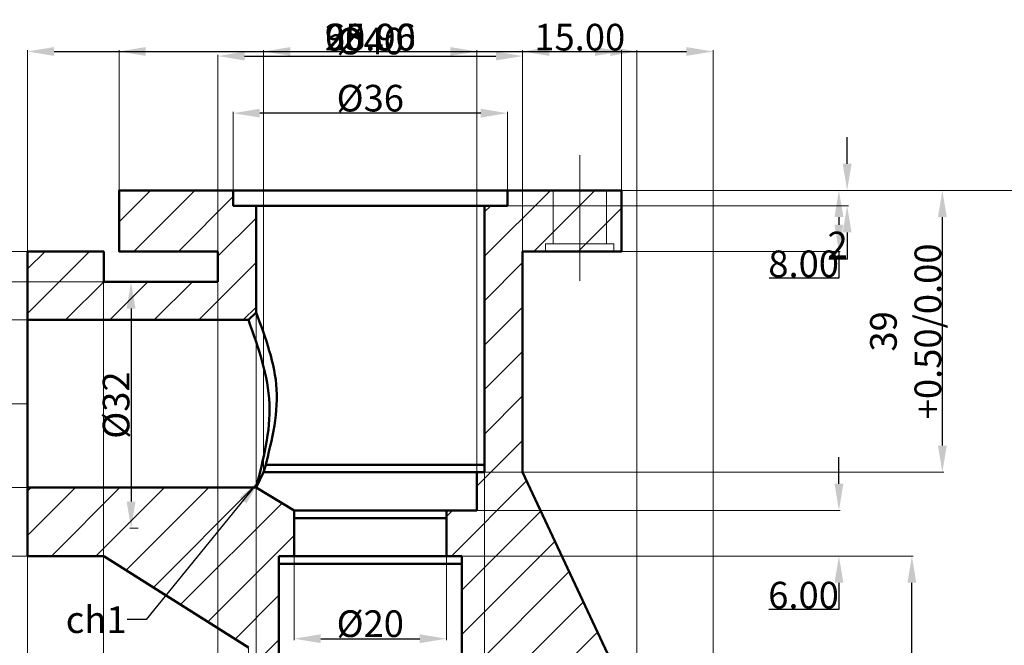
# Model space of a CAD drawing. Units: millimetres. Extents: x 75 to 489, y 21 to 350.
# Tile 4 of 5: x 142 to 271, y 268 to 350. Entities that reach past the tile are written whole.
import ezdxf

# ---------------------------------------------------------------- set-up
doc = ezdxf.new("R2010")
doc.units = ezdxf.units.MM
doc.header["$MEASUREMENT"] = 0
doc.linetypes.add('CENTER', pattern=[50.8, 31.75, -6.35, 6.35, -6.35])
for name, color, linetype, lineweight in [('M-CNTR', 1, 'CENTER', 18), ('M-DIMS', 2, 'Continuous', 25), ('M-HATC', 8, 'Continuous', 18), ('M-OUTL', 7, 'Continuous', 50), ('M-TEXT', 7, 'Continuous', 25), ('M-THRD', 3, 'Continuous', 18)]:
    doc.layers.add(name, color=color, linetype=linetype, lineweight=lineweight)
doc.styles.get("Standard").update_dxf_attribs({"font": 'arial.ttf'})
doc.dimstyles.get("Standard").update_dxf_attribs({"dimtxt": 3.5, "dimasz": 3.5, "dimexe": 0.18, "dimexo": 0.0625, "dimgap": 0.09, "dimtad": 1, "dimtoh": 1, "dimdec": 0, "dimzin": 0, "dimdsep": 46, "dimtxsty": 'Standard', "dimcen": 0.09, "dimclrd": 2, "dimclre": 251, "dimadec": 0, "dimazin": 0, "dimtfac": 1, "dimtdec": 0, "dimtofl": 0, "dimtmove": 0, "dimatfit": 3, "dimfxl": 1, "dimtolj": 1, "dimtzin": 0, "dimlwe": 5, "dimarcsym": 0})

# ---------------------------------------------------------------- blocks, each defined once
blk = doc.blocks.new('*D21')
at = {"layer": 'Defpoints', "color": 0, "transparency": 16777216}
for p in [(169.9, 337.5), (169.9, 327.35), (205.9, 327.35)]:
    blk.add_point(p, dxfattribs=at)
at = {"layer": 'M-DIMS', "color": 0, "lineweight": 5, "transparency": 16777216}
for p, q in [((169.9, 327.41), (169.9, 337.68)), ((205.9, 327.41), (205.9, 337.68))]:
    blk.add_line(p, q, dxfattribs=at)
at = {"layer": 'M-DIMS', "color": 0, "lineweight": -2, "transparency": 16777216}
blk.add_line((202.4, 337.5), (173.4, 337.5), dxfattribs=at)
at = {"layer": 'M-DIMS', "color": 0, "transparency": 16777216}
for points in [[(173.4, 338.08), (173.4, 336.92), (169.9, 337.5)], [(202.4, 338.08), (202.4, 336.92), (205.9, 337.5)]]:
    blk.add_solid(points, dxfattribs=at)
at = {"layer": 'M-DIMS', "color": 0, "transparency": 16777216, "insert": (187.9, 339.47), "char_height": 3.5, "attachment_point": 5}
blk.add_mtext('\\A1;%%C36', dxfattribs=at)
blk = doc.blocks.new('*D22')
at = {"layer": 'Defpoints', "color": 0, "transparency": 16777216}
for p in [(207.9, 345), (167.9, 319.35), (207.9, 319.35)]:
    blk.add_point(p, dxfattribs=at)
at = {"layer": 'M-DIMS', "color": 0, "lineweight": 5, "transparency": 16777216}
for p, q in [((167.9, 319.41), (167.9, 345.18)), ((207.9, 319.41), (207.9, 345.18))]:
    blk.add_line(p, q, dxfattribs=at)
at = {"layer": 'M-DIMS', "color": 0, "lineweight": -2, "transparency": 16777216}
blk.add_line((171.4, 345), (204.4, 345), dxfattribs=at)
at = {"layer": 'M-DIMS', "color": 0, "transparency": 16777216}
for points in [[(171.4, 345.58), (171.4, 344.42), (167.9, 345)], [(204.4, 345.58), (204.4, 344.42), (207.9, 345)]]:
    blk.add_solid(points, dxfattribs=at)
at = {"layer": 'M-DIMS', "color": 0, "transparency": 16777216, "insert": (187.9, 346.97), "char_height": 3.5, "attachment_point": 5}
blk.add_mtext('\\A1;%%C40', dxfattribs=at)
blk = doc.blocks.new('*D23')
at = {"layer": 'Defpoints', "color": 0, "transparency": 16777216}
for p in [(157.5, 315.35), (156.5, 283), (157.5, 283)]:
    blk.add_point(p, dxfattribs=at)
at = {"layer": 'M-DIMS', "color": 0, "lineweight": 5, "transparency": 16777216}
for p, q in [((157.44, 315.35), (156.32, 315.35)), ((157.44, 283), (156.32, 283))]:
    blk.add_line(p, q, dxfattribs=at)
at = {"layer": 'M-DIMS', "color": 0, "lineweight": -2, "transparency": 16777216}
blk.add_line((156.5, 311.85), (156.5, 286.5), dxfattribs=at)
at = {"layer": 'M-DIMS', "color": 0, "transparency": 16777216}
for points in [[(155.92, 311.85), (157.08, 311.85), (156.5, 315.35)], [(155.92, 286.5), (157.08, 286.5), (156.5, 283)]]:
    blk.add_solid(points, dxfattribs=at)
at = {"layer": 'M-DIMS', "color": 0, "transparency": 16777216, "insert": (154.53, 299.17), "char_height": 3.5, "attachment_point": 5, "rotation": 90}
blk.add_mtext('\\A1;%%C32', dxfattribs=at)
blk = doc.blocks.new('*D24')
at = {"layer": 'Defpoints', "color": 0, "transparency": 16777216}
for p in [(133, 310.35), (142.9, 310.35), (142.9, 288.35)]:
    blk.add_point(p, dxfattribs=at)
at = {"layer": 'M-DIMS', "color": 0, "lineweight": 5, "transparency": 16777216}
for p, q in [((142.84, 310.35), (132.82, 310.35)), ((142.84, 288.35), (132.82, 288.35))]:
    blk.add_line(p, q, dxfattribs=at)
at = {"layer": 'M-DIMS', "color": 0, "lineweight": -2, "transparency": 16777216}
blk.add_line((133, 291.85), (133, 306.85), dxfattribs=at)
at = {"layer": 'M-DIMS', "color": 0, "transparency": 16777216}
for points in [[(132.42, 306.85), (133.58, 306.85), (133, 310.35)], [(132.42, 291.85), (133.58, 291.85), (133, 288.35)]]:
    blk.add_solid(points, dxfattribs=at)
at = {"layer": 'M-DIMS', "color": 0, "transparency": 16777216, "insert": (131.03, 299.35), "char_height": 3.5, "attachment_point": 5, "rotation": 90}
blk.add_mtext('\\A1;%%C22', dxfattribs=at)
blk = doc.blocks.new('*D25')
at = {"layer": 'Defpoints', "color": 0, "transparency": 16777216}
for p in [(142.9, 299.35), (125.5, 241.35), (232.9, 241.35)]:
    blk.add_point(p, dxfattribs=at)
at = {"layer": 'M-DIMS', "color": 0, "lineweight": 5, "transparency": 16777216}
for p, q in [((142.84, 299.35), (125.32, 299.35)), ((232.84, 241.35), (125.32, 241.35))]:
    blk.add_line(p, q, dxfattribs=at)
at = {"layer": 'M-DIMS', "color": 0, "lineweight": -2, "transparency": 16777216}
blk.add_line((125.5, 295.85), (125.5, 244.85), dxfattribs=at)
at = {"layer": 'M-DIMS', "color": 0, "transparency": 16777216}
for points in [[(124.92, 295.85), (126.08, 295.85), (125.5, 299.35)], [(124.92, 244.85), (126.08, 244.85), (125.5, 241.35)]]:
    blk.add_solid(points, dxfattribs=at)
at = {"layer": 'M-DIMS', "color": 0, "transparency": 16777216, "insert": (123.62, 270.35), "char_height": 3.5, "attachment_point": 5, "rotation": 90}
blk.add_mtext('\\A1;58', dxfattribs=at)
blk = doc.blocks.new('*D26')
at = {"layer": 'Defpoints', "color": 0, "transparency": 16777216}
for p in [(117, 299.35), (142.9, 299.35), (155.4, 209.35)]:
    blk.add_point(p, dxfattribs=at)
at = {"layer": 'M-DIMS', "color": 0, "lineweight": 5, "transparency": 16777216}
for p, q in [((142.84, 299.35), (116.82, 299.35)), ((155.34, 209.35), (116.82, 209.35))]:
    blk.add_line(p, q, dxfattribs=at)
at = {"layer": 'M-DIMS', "color": 0, "lineweight": -2, "transparency": 16777216}
blk.add_line((117, 212.85), (117, 295.85), dxfattribs=at)
at = {"layer": 'M-DIMS', "color": 0, "transparency": 16777216}
for points in [[(116.42, 295.85), (117.58, 295.85), (117, 299.35)], [(116.42, 212.85), (117.58, 212.85), (117, 209.35)]]:
    blk.add_solid(points, dxfattribs=at)
at = {"layer": 'M-DIMS', "color": 0, "transparency": 16777216, "insert": (115.12, 254.35), "char_height": 3.5, "attachment_point": 5, "rotation": 90}
blk.add_mtext('\\A1;90', dxfattribs=at)
blk = doc.blocks.new('*D31')
at = {"layer": 'Defpoints', "color": 0, "transparency": 16777216}
for p in [(199.9, 279.35), (259, 279.35), (220.4, 209.35)]:
    blk.add_point(p, dxfattribs=at)
at = {"layer": 'M-DIMS', "color": 0, "lineweight": 5, "transparency": 16777216}
for p, q in [((199.97, 279.35), (259.18, 279.35)), ((220.47, 209.35), (259.18, 209.35))]:
    blk.add_line(p, q, dxfattribs=at)
at = {"layer": 'M-DIMS', "color": 0, "lineweight": -2, "transparency": 16777216}
blk.add_line((259, 212.85), (259, 275.85), dxfattribs=at)
at = {"layer": 'M-DIMS', "color": 0, "transparency": 16777216}
for points in [[(258.42, 275.85), (259.58, 275.85), (259, 279.35)], [(258.42, 212.85), (259.58, 212.85), (259, 209.35)]]:
    blk.add_solid(points, dxfattribs=at)
at = {"layer": 'M-DIMS', "color": 0, "transparency": 16777216, "insert": (257.12, 244.35), "char_height": 3.5, "attachment_point": 5, "rotation": 90}
blk.add_mtext('\\A1;70', dxfattribs=at)
blk = doc.blocks.new('*D32')
at = {"layer": 'Defpoints', "color": 0, "transparency": 16777216}
for p in [(177.9, 279.35), (197.9, 279.35), (197.9, 268.5)]:
    blk.add_point(p, dxfattribs=at)
at = {"layer": 'M-DIMS', "color": 0, "lineweight": 5, "transparency": 16777216}
for p, q in [((177.9, 279.28), (177.9, 268.32)), ((197.9, 279.28), (197.9, 268.32))]:
    blk.add_line(p, q, dxfattribs=at)
at = {"layer": 'M-DIMS', "color": 0, "lineweight": -2, "transparency": 16777216}
blk.add_line((181.4, 268.5), (194.4, 268.5), dxfattribs=at)
at = {"layer": 'M-DIMS', "color": 0, "transparency": 16777216}
for points in [[(181.4, 269.08), (181.4, 267.92), (177.9, 268.5)], [(194.4, 269.08), (194.4, 267.92), (197.9, 268.5)]]:
    blk.add_solid(points, dxfattribs=at)
at = {"layer": 'M-DIMS', "color": 0, "transparency": 16777216, "insert": (187.9, 270.47), "char_height": 3.5, "attachment_point": 5}
blk.add_mtext('\\A1;%%C20', dxfattribs=at)
blk = doc.blocks.new('*D33')
at = {"layer": 'Defpoints', "color": 0, "transparency": 16777216}
for p in [(205.9, 327.35), (205.9, 325.35), (250.5, 325.35)]:
    blk.add_point(p, dxfattribs=at)
at = {"layer": 'M-DIMS', "color": 0, "lineweight": -2, "transparency": 16777216}
for p, q in [((250.5, 330.85), (250.5, 334.35)), ((250.5, 321.85), (250.5, 318.35)), ((250.5, 318.35), (248.09, 318.35))]:
    blk.add_line(p, q, dxfattribs=at)
at = {"layer": 'M-DIMS', "color": 0, "lineweight": 5, "transparency": 16777216}
for p, q in [((205.97, 327.35), (250.68, 327.35)), ((205.97, 325.35), (250.68, 325.35))]:
    blk.add_line(p, q, dxfattribs=at)
at = {"layer": 'M-DIMS', "color": 0, "transparency": 16777216}
for points in [[(249.92, 330.85), (251.08, 330.85), (250.5, 327.35)], [(249.92, 321.85), (251.08, 321.85), (250.5, 325.35)]]:
    blk.add_solid(points, dxfattribs=at)
at = {"layer": 'M-DIMS', "color": 0, "transparency": 16777216, "insert": (249.25, 320.19), "char_height": 3.5, "attachment_point": 5}
blk.add_mtext('\\A1;2', dxfattribs=at)
blk = doc.blocks.new('*D34')
at = {"layer": 'Defpoints', "color": 0, "transparency": 16777216}
for p in [(205.9, 327.35), (263, 327.35), (202.9, 290.35)]:
    blk.add_point(p, dxfattribs=at)
at = {"layer": 'M-DIMS', "color": 0, "lineweight": 5, "transparency": 16777216}
for p, q in [((205.97, 327.35), (263.18, 327.35)), ((202.97, 290.35), (263.18, 290.35))]:
    blk.add_line(p, q, dxfattribs=at)
at = {"layer": 'M-DIMS', "color": 0, "lineweight": -2, "transparency": 16777216}
blk.add_line((263, 293.85), (263, 323.85), dxfattribs=at)
at = {"layer": 'M-DIMS', "color": 0, "transparency": 16777216}
for points in [[(262.42, 323.85), (263.58, 323.85), (263, 327.35)], [(262.42, 293.85), (263.58, 293.85), (263, 290.35)]]:
    blk.add_solid(points, dxfattribs=at)
at = {"layer": 'M-DIMS', "color": 0, "transparency": 16777216, "insert": (258.18, 308.85), "char_height": 3.5, "attachment_point": 5, "rotation": 90}
blk.add_mtext('\\A1;39\\P+0.50/0.00', dxfattribs=at)
blk = doc.blocks.new('*D35')
at = {"layer": 'Defpoints', "color": 0, "transparency": 16777216}
for p in [(220.88, 327.35), (259, 209.35), (279.5, 209.35)]:
    blk.add_point(p, dxfattribs=at)
at = {"layer": 'M-DIMS', "color": 0, "lineweight": 5, "transparency": 16777216}
for p, q in [((220.95, 327.35), (279.68, 327.35)), ((259.06, 209.35), (279.68, 209.35))]:
    blk.add_line(p, q, dxfattribs=at)
at = {"layer": 'M-DIMS', "color": 0, "lineweight": -2, "transparency": 16777216}
blk.add_line((279.5, 323.85), (279.5, 212.85), dxfattribs=at)
at = {"layer": 'M-DIMS', "color": 0, "transparency": 16777216}
for points in [[(278.92, 323.85), (280.08, 323.85), (279.5, 327.35)], [(278.92, 212.85), (280.08, 212.85), (279.5, 209.35)]]:
    blk.add_solid(points, dxfattribs=at)
at = {"layer": 'M-DIMS', "color": 0, "transparency": 16777216, "insert": (277.62, 268.35), "char_height": 3.5, "attachment_point": 5, "rotation": 90}
blk.add_mtext('\\A1;118', dxfattribs=at)
blk = doc.blocks.new('*D44')
at = {"layer": 'Defpoints', "color": 0, "transparency": 16777216}
for p in [(232.9, 345.6), (142.9, 319.35), (232.9, 258.35)]:
    blk.add_point(p, dxfattribs=at)
at = {"layer": 'M-DIMS', "color": 251, "lineweight": 5, "transparency": 16777216}
for p, q in [((142.9, 319.41), (142.9, 345.78)), ((232.9, 258.41), (232.9, 345.78))]:
    blk.add_line(p, q, dxfattribs=at)
at = {"layer": 'M-DIMS', "color": 2, "lineweight": -2, "transparency": 16777216}
blk.add_line((146.4, 345.6), (229.4, 345.6), dxfattribs=at)
at = {"layer": 'M-DIMS', "color": 2, "transparency": 16777216}
for points in [[(146.4, 346.18), (146.4, 345.02), (142.9, 345.6)], [(229.4, 346.18), (229.4, 345.02), (232.9, 345.6)]]:
    blk.add_solid(points, dxfattribs=at)
at = {"layer": 'M-DIMS', "color": 0, "transparency": 16777216, "insert": (187.9, 347.48), "char_height": 3.5, "attachment_point": 5}
blk.add_mtext('\\A1;90.00', dxfattribs=at)
blk = doc.blocks.new('*D45')
at = {"layer": 'Defpoints', "color": 0, "transparency": 16777216}
for p in [(220.88, 345.6), (154.92, 327.35), (220.88, 327.35)]:
    blk.add_point(p, dxfattribs=at)
at = {"layer": 'M-DIMS', "color": 251, "lineweight": 5, "transparency": 16777216}
for p, q in [((154.92, 327.41), (154.92, 345.78)), ((220.88, 327.41), (220.88, 345.78))]:
    blk.add_line(p, q, dxfattribs=at)
at = {"layer": 'M-DIMS', "color": 2, "lineweight": -2, "transparency": 16777216}
blk.add_line((158.42, 345.6), (217.38, 345.6), dxfattribs=at)
at = {"layer": 'M-DIMS', "color": 2, "transparency": 16777216}
for points in [[(158.42, 346.18), (158.42, 345.02), (154.92, 345.6)], [(217.38, 346.18), (217.38, 345.02), (220.88, 345.6)]]:
    blk.add_solid(points, dxfattribs=at)
at = {"layer": 'M-DIMS', "color": 0, "transparency": 16777216, "insert": (187.9, 347.48), "char_height": 3.5, "attachment_point": 5}
blk.add_mtext('\\A1;65.96', dxfattribs=at)
blk = doc.blocks.new('*D46')
at = {"layer": 'Defpoints', "color": 0, "transparency": 16777216}
for p in [(220.88, 327.35), (220.88, 319.35), (249.42, 319.35)]:
    blk.add_point(p, dxfattribs=at)
at = {"layer": 'M-DIMS', "color": 251, "lineweight": 5, "transparency": 16777216}
for p, q in [((220.95, 327.35), (249.6, 327.35)), ((220.95, 319.35), (249.6, 319.35))]:
    blk.add_line(p, q, dxfattribs=at)
at = {"layer": 'M-DIMS', "color": 2, "lineweight": -2, "transparency": 16777216}
for p, q in [((249.42, 323.85), (249.42, 322.85)), ((249.42, 319.35), (249.42, 315.85)), ((249.42, 315.85), (240.25, 315.85))]:
    blk.add_line(p, q, dxfattribs=at)
at = {"layer": 'M-DIMS', "color": 2, "transparency": 16777216}
for points in [[(248.84, 323.85), (250.01, 323.85), (249.42, 327.35)], [(248.84, 322.85), (250.01, 322.85), (249.42, 319.35)]]:
    blk.add_solid(points, dxfattribs=at)
at = {"layer": 'M-DIMS', "color": 0, "transparency": 16777216, "insert": (244.79, 317.72), "char_height": 3.5, "attachment_point": 5}
blk.add_mtext('\\A1;8.00', dxfattribs=at)
blk = doc.blocks.new('*D49')
at = {"layer": 'Defpoints', "color": 0, "transparency": 16777216}
for p in [(142.9, 319.35), (84.4, 279.35), (142.9, 279.35)]:
    blk.add_point(p, dxfattribs=at)
at = {"layer": 'M-DIMS', "color": 251, "lineweight": 5, "transparency": 16777216}
for p, q in [((142.84, 319.35), (84.22, 319.35)), ((142.84, 279.35), (84.22, 279.35))]:
    blk.add_line(p, q, dxfattribs=at)
at = {"layer": 'M-DIMS', "color": 2, "lineweight": -2, "transparency": 16777216}
blk.add_line((84.4, 315.85), (84.4, 282.85), dxfattribs=at)
at = {"layer": 'M-DIMS', "color": 2, "transparency": 16777216}
for points in [[(83.82, 315.85), (84.98, 315.85), (84.4, 319.35)], [(83.82, 282.85), (84.98, 282.85), (84.4, 279.35)]]:
    blk.add_solid(points, dxfattribs=at)
at = {"layer": 'M-DIMS', "color": 0, "transparency": 16777216, "insert": (82.52, 299.35), "char_height": 3.5, "attachment_point": 5, "rotation": 90}
blk.add_mtext('\\A1;40.00', dxfattribs=at)
blk = doc.blocks.new('*D50')
at = {"layer": 'Defpoints', "color": 0, "transparency": 16777216}
for p in [(142.9, 279.35), (152.9, 279.35), (152.9, 189.4)]:
    blk.add_point(p, dxfattribs=at)
at = {"layer": 'M-DIMS', "color": 251, "lineweight": 5, "transparency": 16777216}
for p, q in [((142.9, 279.28), (142.9, 189.22)), ((152.9, 279.28), (152.9, 189.22))]:
    blk.add_line(p, q, dxfattribs=at)
at = {"layer": 'M-DIMS', "color": 2, "lineweight": -2, "transparency": 16777216}
for p, q in [((146.4, 189.4), (149.4, 189.4)), ((152.9, 189.4), (168.05, 189.4))]:
    blk.add_line(p, q, dxfattribs=at)
at = {"layer": 'M-DIMS', "color": 2, "transparency": 16777216}
for points in [[(146.4, 189.98), (146.4, 188.82), (142.9, 189.4)], [(149.4, 189.98), (149.4, 188.82), (152.9, 189.4)]]:
    blk.add_solid(points, dxfattribs=at)
at = {"layer": 'M-DIMS', "color": 0, "transparency": 16777216, "insert": (162.23, 191.28), "char_height": 3.5, "attachment_point": 5}
blk.add_mtext('\\A1;10.00', dxfattribs=at)
blk = doc.blocks.new('*D51')
at = {"layer": 'Defpoints', "color": 0, "transparency": 16777216}
for p in [(142.9, 279.35), (171.9, 267.35), (171.9, 189.4)]:
    blk.add_point(p, dxfattribs=at)
at = {"layer": 'M-DIMS', "color": 251, "lineweight": 5, "transparency": 16777216}
for p, q in [((142.9, 279.28), (142.9, 189.22)), ((171.9, 267.28), (171.9, 189.22))]:
    blk.add_line(p, q, dxfattribs=at)
at = {"layer": 'M-DIMS', "color": 2, "lineweight": -2, "transparency": 16777216}
blk.add_line((146.4, 189.4), (168.4, 189.4), dxfattribs=at)
at = {"layer": 'M-DIMS', "color": 2, "transparency": 16777216}
for points in [[(146.4, 189.98), (146.4, 188.82), (142.9, 189.4)], [(168.4, 189.98), (168.4, 188.82), (171.9, 189.4)]]:
    blk.add_solid(points, dxfattribs=at)
at = {"layer": 'M-DIMS', "color": 0, "transparency": 16777216, "insert": (157.4, 191.28), "char_height": 3.5, "attachment_point": 5}
blk.add_mtext('\\A1;29.00', dxfattribs=at)
blk = doc.blocks.new('*D52')
at = {"layer": 'Defpoints', "color": 0, "transparency": 16777216}
for p in [(222.9, 345.6), (207.9, 290.35), (222.9, 258.35)]:
    blk.add_point(p, dxfattribs=at)
at = {"layer": 'M-DIMS', "color": 251, "lineweight": 5, "transparency": 16777216}
for p, q in [((207.9, 290.41), (207.9, 345.78)), ((222.9, 258.41), (222.9, 345.78))]:
    blk.add_line(p, q, dxfattribs=at)
at = {"layer": 'M-DIMS', "color": 2, "lineweight": -2, "transparency": 16777216}
blk.add_line((211.4, 345.6), (219.4, 345.6), dxfattribs=at)
at = {"layer": 'M-DIMS', "color": 2, "transparency": 16777216}
for points in [[(211.4, 346.18), (211.4, 345.02), (207.9, 345.6)], [(219.4, 346.18), (219.4, 345.02), (222.9, 345.6)]]:
    blk.add_solid(points, dxfattribs=at)
at = {"layer": 'M-DIMS', "color": 0, "transparency": 16777216, "insert": (215.4, 347.48), "char_height": 3.5, "attachment_point": 5}
blk.add_mtext('\\A1;15.00', dxfattribs=at)
blk = doc.blocks.new('*D53')
at = {"layer": 'Defpoints', "color": 0, "transparency": 16777216}
for p in [(152.9, 315.35), (167.9, 315.35), (167.9, 189.4)]:
    blk.add_point(p, dxfattribs=at)
at = {"layer": 'M-DIMS', "color": 251, "lineweight": 5, "transparency": 16777216}
for p, q in [((152.9, 315.28), (152.9, 189.22)), ((167.9, 315.28), (167.9, 189.22))]:
    blk.add_line(p, q, dxfattribs=at)
at = {"layer": 'M-DIMS', "color": 2, "lineweight": -2, "transparency": 16777216}
blk.add_line((156.4, 189.4), (164.4, 189.4), dxfattribs=at)
at = {"layer": 'M-DIMS', "color": 2, "transparency": 16777216}
for points in [[(156.4, 189.98), (156.4, 188.82), (152.9, 189.4)], [(164.4, 189.98), (164.4, 188.82), (167.9, 189.4)]]:
    blk.add_solid(points, dxfattribs=at)
at = {"layer": 'M-DIMS', "color": 0, "transparency": 16777216, "insert": (160.4, 191.28), "char_height": 3.5, "attachment_point": 5}
blk.add_mtext('\\A1;15.00', dxfattribs=at)
blk = doc.blocks.new('*D57')
at = {"layer": 'Defpoints', "color": 0, "transparency": 16777216}
for p in [(172.9, 325.35), (202.9, 325.35), (202.9, 189.4)]:
    blk.add_point(p, dxfattribs=at)
at = {"layer": 'M-DIMS', "color": 251, "lineweight": 5, "transparency": 16777216}
for p, q in [((172.9, 325.28), (172.9, 189.22)), ((202.9, 325.28), (202.9, 189.22))]:
    blk.add_line(p, q, dxfattribs=at)
at = {"layer": 'M-DIMS', "color": 2, "lineweight": -2, "transparency": 16777216}
blk.add_line((176.4, 189.4), (199.4, 189.4), dxfattribs=at)
at = {"layer": 'M-DIMS', "color": 2, "transparency": 16777216}
for points in [[(176.4, 189.98), (176.4, 188.82), (172.9, 189.4)], [(199.4, 189.98), (199.4, 188.82), (202.9, 189.4)]]:
    blk.add_solid(points, dxfattribs=at)
at = {"layer": 'M-DIMS', "color": 0, "transparency": 16777216, "insert": (187.9, 191.28), "char_height": 3.5, "attachment_point": 5}
blk.add_mtext('\\A1;30.00', dxfattribs=at)
blk = doc.blocks.new('*D58')
at = {"layer": 'Defpoints', "color": 0, "transparency": 16777216}
for p in [(201.9, 345.6), (173.9, 290.35), (201.9, 290.35)]:
    blk.add_point(p, dxfattribs=at)
at = {"layer": 'M-DIMS', "color": 251, "lineweight": 5, "transparency": 16777216}
for p, q in [((173.9, 290.41), (173.9, 345.78)), ((201.9, 290.41), (201.9, 345.78))]:
    blk.add_line(p, q, dxfattribs=at)
at = {"layer": 'M-DIMS', "color": 2, "lineweight": -2, "transparency": 16777216}
blk.add_line((177.4, 345.6), (198.4, 345.6), dxfattribs=at)
at = {"layer": 'M-DIMS', "color": 2, "transparency": 16777216}
for points in [[(177.4, 346.18), (177.4, 345.02), (173.9, 345.6)], [(198.4, 346.18), (198.4, 345.02), (201.9, 345.6)]]:
    blk.add_solid(points, dxfattribs=at)
at = {"layer": 'M-DIMS', "color": 0, "transparency": 16777216, "insert": (187.9, 347.48), "char_height": 3.5, "attachment_point": 5}
blk.add_mtext('\\A1;28.00', dxfattribs=at)
blk = doc.blocks.new('*D59')
at = {"layer": 'Defpoints', "color": 0, "transparency": 16777216}
for p in [(197.9, 285.35), (197.9, 279.35), (249.42, 279.35)]:
    blk.add_point(p, dxfattribs=at)
at = {"layer": 'M-DIMS', "color": 2, "lineweight": -2, "transparency": 16777216}
for p, q in [((249.42, 288.85), (249.42, 292.35)), ((249.42, 275.85), (249.42, 272.35)), ((249.42, 272.35), (240.23, 272.35))]:
    blk.add_line(p, q, dxfattribs=at)
at = {"layer": 'M-DIMS', "color": 251, "lineweight": 5, "transparency": 16777216}
for p, q in [((197.97, 285.35), (249.6, 285.35)), ((197.97, 279.35), (249.6, 279.35))]:
    blk.add_line(p, q, dxfattribs=at)
at = {"layer": 'M-DIMS', "color": 2, "transparency": 16777216}
for points in [[(248.84, 288.85), (250.01, 288.85), (249.42, 285.35)], [(248.84, 275.85), (250.01, 275.85), (249.42, 279.35)]]:
    blk.add_solid(points, dxfattribs=at)
at = {"layer": 'M-DIMS', "color": 0, "transparency": 16777216, "insert": (244.78, 274.22), "char_height": 3.5, "attachment_point": 5}
blk.add_mtext('\\A1;6.00', dxfattribs=at)
blk = doc.blocks.new('*D60')
at = {"layer": 'Defpoints', "color": 0, "transparency": 16777216}
for p in [(152.9, 319.35), (84.4, 315.35), (152.9, 315.35)]:
    blk.add_point(p, dxfattribs=at)
at = {"layer": 'M-DIMS', "color": 2, "lineweight": -2, "transparency": 16777216}
for p, q in [((84.4, 322.85), (84.4, 326.35)), ((84.4, 311.85), (84.4, 308.35)), ((84.4, 308.35), (75.09, 308.35))]:
    blk.add_line(p, q, dxfattribs=at)
at = {"layer": 'M-DIMS', "color": 251, "lineweight": 5, "transparency": 16777216}
for p, q in [((152.84, 319.35), (84.22, 319.35)), ((152.84, 315.35), (84.22, 315.35))]:
    blk.add_line(p, q, dxfattribs=at)
at = {"layer": 'M-DIMS', "color": 2, "transparency": 16777216}
for points in [[(83.82, 322.85), (84.98, 322.85), (84.4, 319.35)], [(83.82, 311.85), (84.98, 311.85), (84.4, 315.35)]]:
    blk.add_solid(points, dxfattribs=at)
at = {"layer": 'M-DIMS', "color": 0, "transparency": 16777216, "insert": (79.7, 310.22), "char_height": 3.5, "attachment_point": 5}
blk.add_mtext('\\A1;4.00', dxfattribs=at)

msp = doc.modelspace()

# ---------------------------------------------------------------- hatches: boundary and pattern name
at = {"layer": 'M-HATC'}
h = msp.add_hatch(dxfattribs=at)
h.set_pattern_fill('ANSI31', color=256, scale=33)
h.set_pattern_definition([(45, (-570, 152.5), (-2.916815, 2.916815), [])])
h.paths.add_polyline_path([(172.904, 325.347), (169.904, 325.347), (169.904, 327.347), (154.923, 327.347), (154.923, 319.347), (167.904, 319.347), (167.904, 315.347), (152.904, 315.347), (152.904, 319.347), (142.904, 319.347), (142.904, 310.347), (172.904, 310.347)])
h.paths.add_polyline_path([(220.885, 327.347), (205.904, 327.347), (205.904, 325.347), (202.904, 325.347), (202.904, 290.347), (201.904, 290.347), (201.904, 285.347), (197.904, 285.347), (197.904, 279.347), (199.904, 279.347), (199.904, 250.347), (232.904, 250.347), (232.904, 258.347), (222.904, 258.347), (207.904, 290.347), (207.904, 319.347), (220.885, 319.347)])
h.paths.add_polyline_path([(232.781, 232.347), (199.781, 232.347), (199.904, 209.347), (220.404, 209.347), (220.404, 219.347), (203.904, 219.347), (203.904, 227.347), (222.904, 227.347), (222.904, 224.347), (232.904, 224.347)])
h.paths.add_polyline_path([(175.904, 279.347), (177.904, 279.347), (177.904, 285.347), (172.904, 288.347), (142.904, 288.347), (142.904, 279.347), (152.904, 279.347), (171.904, 267.347), (171.904, 219.347), (155.404, 219.347), (155.404, 209.347), (175.904, 209.347)])

# ---------------------------------------------------------------- linework, layer by layer
at = {"layer": 'M-CNTR'}
msp.add_line((215.404, 315.5), (215.404, 332), dxfattribs=at)
at = {"layer": 'M-OUTL'}
for p, q in [((172.904, 311.347), (172.904, 325.347)), ((202.904, 290.347), (202.904, 325.347)), ((142.904, 279.347), (142.904, 319.347)), ((142.904, 319.347), (152.904, 319.347)), ((152.904, 319.347), (152.904, 315.347)), ((167.904, 315.347), (167.904, 319.347)), ((207.904, 290.347), (207.904, 319.347)), ((152.904, 315.347), (167.904, 315.347)), ((142.904, 310.347), (171.904, 310.347)), ((171.904, 310.347), (172.904, 311.347)), ((174.146, 291.347), (202.904, 291.347)), ((172.904, 288.347), (173.904, 290.347)), ((173.904, 290.347), (202.904, 290.347)), ((201.904, 285.347), (201.904, 290.347)), ((222.904, 258.347), (207.904, 290.347)), ((142.904, 288.347), (172.904, 288.347)), ((172.904, 288.347), (177.904, 285.347)), ((177.904, 285.347), (197.904, 285.347)), ((177.904, 285.347), (177.904, 279.347)), ((197.904, 285.347), (197.904, 279.347)), ((197.904, 285.347), (201.904, 285.347)), ((177.904, 284.347), (197.904, 284.347)), ((142.904, 279.347), (152.904, 279.347)), ((152.904, 279.347), (171.904, 267.347)), ((175.904, 279.347), (199.904, 279.347)), ((175.904, 279.347), (175.904, 209.347)), ((199.904, 251.347), (199.904, 279.347)), ((175.904, 278.347), (199.904, 278.347))]:
    msp.add_line(p, q, dxfattribs=at)
for points in [[(167.904, 319.347), (154.923, 319.347), (154.923, 327.347), (172.904, 327.347)], [(207.904, 319.347), (220.885, 319.347), (220.885, 327.347), (202.904, 327.347)]]:
    msp.add_lwpolyline(points, dxfattribs=at)
msp.add_lwpolyline([(169.904, 327.347), (205.904, 327.347), (205.904, 325.347), (169.904, 325.347)], close=True, dxfattribs=at)
for points, knots in [([(171.904, 310.347), (173.209, 306.697), (175.797, 299.462), (173.862, 292.03), (172.904, 288.347)], [0, 0, 0, 0, 11.3422338, 22.482965, 22.482965, 22.482965, 22.482965]), ([(172.904, 311.347), (174.156, 307.99), (176.722, 301.108), (174.858, 293.992), (173.904, 290.347)], [0, 0, 0, 0, 10.4822015, 21.4863427, 21.4863427, 21.4863427, 21.4863427])]:
    msp.add_open_spline(points, degree=3, knots=knots, dxfattribs=at)
at = {"layer": 'M-THRD'}
for p, q in [((211.904, 320.347), (211.904, 327.347)), ((218.904, 320.347), (218.904, 327.347)), ((210.923, 320.347), (219.885, 320.347)), ((210.923, 320.347), (210.923, 319.347)), ((219.885, 320.347), (219.885, 319.347))]:
    msp.add_line(p, q, dxfattribs=at)

# ---------------------------------------------------------------- texts
at = {"layer": 'M-TEXT', "insert": (155.91, 269.25), "char_height": 3.5, "attachment_point": 9}
msp.add_mtext('\\A1;ch1', dxfattribs=at)

# ---------------------------------------------------------------- dimensions: what is measured, and where the dimension line sits
at = {"layer": 'M-DIMS'}
for base, p1, p2, picture, middle in [((232.904, 345.6), (142.904, 319.347), (232.904, 258.347), '*D44', (187.904, 347.477)), ((220.885, 345.6), (154.923, 327.347), (220.885, 327.347), '*D45', (187.904, 347.477)), ((201.904, 345.6), (173.904, 290.347), (201.904, 290.347), '*D58', (187.904, 347.477)), ((222.904, 345.6), (207.904, 290.347), (222.904, 258.347), '*D52', (215.404, 347.477)), ((202.904, 189.4), (172.904, 325.347), (202.904, 325.347), '*D57', (187.904, 191.278)), ((167.904, 189.4), (152.904, 315.347), (167.904, 315.347), '*D53', (160.404, 191.277)), ((152.904, 189.4), (142.904, 279.347), (152.904, 279.347), '*D50', (162.229, 191.277)), ((171.904, 189.4), (142.904, 279.347), (171.904, 267.347), '*D51', (157.404, 191.277))]:
    dim = msp.add_linear_dim(base=base, p1=p1, p2=p2, dimstyle='Standard', override={"dimdec": 2, "dimlfac": 1, "dimrnd": 0, "dimzin": 0, "dimdsep": 46, "dimlunit": 2}, dxfattribs=at)
    dim.commit()
    dim.dimension.update_dxf_attribs({"geometry": picture, "text_midpoint": middle})
for base, p1, p2, picture, middle in [((207.904, 345), (167.904, 319.347), (207.904, 319.347), '*D22', (187.904, 346.975)), ((169.904, 337.5), (205.904, 327.347), (169.904, 327.347), '*D21', (187.904, 339.475)), ((197.904, 268.5), (177.904, 279.347), (197.904, 279.347), '*D32', (187.904, 270.475))]:
    dim = msp.add_linear_dim(base=base, p1=p1, p2=p2, text='%%C<>', dimstyle='Standard', override={"dimclrd": 0, "dimclre": 0, "dimclrt": 0}, dxfattribs=at)
    dim.commit()
    dim.dimension.update_dxf_attribs({"geometry": picture, "text_midpoint": middle})
for base, p1, p2, override, picture, middle in [((250.5, 325.347), (205.904, 327.347), (205.904, 325.347), {"dimclrd": 0, "dimclre": 0, "dimclrt": 0}, '*D33', (249.251, 320.194)), ((279.5, 209.347), (220.885, 327.347), (259, 209.347), {"dimclrd": 0, "dimclre": 0, "dimclrt": 0}, '*D35', (277.623, 268.347)), ((249.423, 319.347), (220.885, 327.347), (220.885, 319.347), {"dimdec": 2, "dimlfac": 1, "dimrnd": 0, "dimzin": 0, "dimdsep": 46, "dimlunit": 2}, '*D46', (244.791, 317.724)), ((84.4, 315.347), (152.904, 319.347), (152.904, 315.347), {"dimdec": 2, "dimlfac": 1, "dimrnd": 0, "dimzin": 0, "dimdsep": 46, "dimlunit": 2}, '*D60', (79.7, 310.224)), ((84.4, 279.347), (142.904, 319.347), (142.904, 279.347), {"dimdec": 2, "dimlfac": 1, "dimrnd": 0, "dimzin": 0, "dimdsep": 46, "dimlunit": 2}, '*D49', (82.523, 299.347)), ((117, 299.347), (155.404, 209.347), (142.904, 299.347), {"dimclrd": 0, "dimclre": 0, "dimclrt": 0}, '*D26', (115.123, 254.347)), ((125.5, 241.347), (142.904, 299.347), (232.904, 241.347), {"dimclrd": 0, "dimclre": 0, "dimclrt": 0}, '*D25', (123.623, 270.347)), ((249.423, 279.347), (197.904, 285.347), (197.904, 279.347), {"dimdec": 2, "dimlfac": 1, "dimrnd": 0, "dimzin": 0, "dimdsep": 46, "dimlunit": 2}, '*D59', (244.784, 274.224)), ((259, 279.347), (220.404, 209.347), (199.904, 279.347), {"dimclrd": 0, "dimclre": 0, "dimclrt": 0}, '*D31', (257.123, 244.347))]:
    dim = msp.add_linear_dim(base=base, p1=p1, p2=p2, angle=90, dimstyle='Standard', override=override, dxfattribs=at)
    dim.commit()
    dim.dimension.update_dxf_attribs({"geometry": picture, "text_midpoint": middle})
for base, p1, p2, text, picture, middle in [((263, 327.347), (202.904, 290.347), (205.904, 327.347), '39\\P+0.50/0.00', '*D34', (258.176, 308.847)), ((156.5, 283), (157.5, 315.347), (157.5, 283), '%%C<>', '*D23', (154.525, 299.174)), ((133, 310.347), (142.904, 288.347), (142.904, 310.347), '%%C<>', '*D24', (131.025, 299.347))]:
    dim = msp.add_linear_dim(base=base, p1=p1, p2=p2, angle=90, text=text, dimstyle='Standard', override={"dimclrd": 0, "dimclre": 0, "dimclrt": 0}, dxfattribs=at)
    dim.commit()
    dim.dimension.update_dxf_attribs({"geometry": picture, "text_midpoint": middle})

# ---------------------------------------------------------------- leaders
at = {"layer": 'M-DIMS', "annotation_type": 0, "has_hookline": 1, "hookline_direction": 1, "text_width": 6.795}
msp.add_leader([(173.404, 289.347), (158.5, 271), (156, 271)], dimstyle='Standard', override={"dimgap": 0.09, "dimtad": 0}, dxfattribs=at)

doc.saveas('drawing.dxf')
